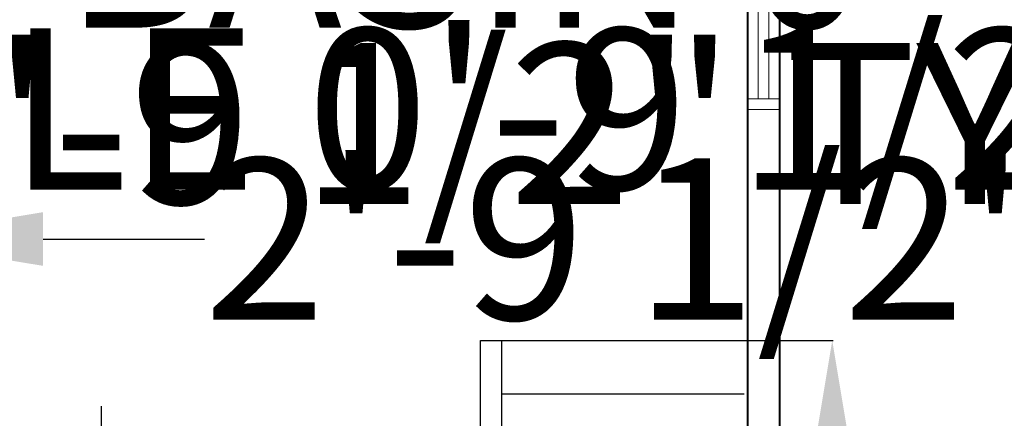
# Model space of a CAD drawing. Units: inches. Extents: x 7323 to 9737, y 2037 to 3322.
# Tile 13 of 19: x 9130 to 9314, y 2337 to 2411. Entities that reach past the tile are written whole.
import ezdxf

# ---------------------------------------------------------------- set-up
doc = ezdxf.new("R2010")
doc.units = ezdxf.units.IN
doc.header["$MEASUREMENT"] = 0
for name, color, linetype, lineweight in [('A-ANNO-DIMS', 2, 'Continuous', 18), ('A-FLOR-STRS', 7, 'Continuous', 25), ('A-GLAZ', 4, 'Continuous', 18), ('A-WALL', 7, 'Continuous', 40)]:
    doc.layers.add(name, color=color, linetype=linetype, lineweight=lineweight)
doc.styles.get("Standard").update_dxf_attribs({"font": 'arial.ttf'})
doc.dimstyles.get("Standard").update_dxf_attribs({"dimtxt": 30.18, "dimasz": 30.18, "dimexe": 0.18, "dimexo": 0.0625, "dimgap": 0.09, "dimtad": 0, "dimtih": 1, "dimtoh": 1, "dimdec": 0, "dimzin": 0, "dimdsep": 46, "dimlunit": 3, "dimtxsty": 'Standard', "dimcen": 0.09, "dimadec": 0, "dimazin": 0, "dimtfac": 1, "dimtdec": 0, "dimtofl": 0, "dimtmove": 0, "dimatfit": 3, "dimfxl": 1, "dimtolj": 1, "dimtzin": 0, "dimarcsym": 0})

# ---------------------------------------------------------------- blocks, each defined once
blk = doc.blocks.new('WIN-48')
for p, q in [((0, 0), (0, 6)), ((2, 0), (2, 6)), ((50, 0), (50, 6)), ((52, 0), (52, 6)), ((2, 4), (50, 4)), ((2, 2), (50, 2))]:
    blk.add_line(p, q)
blk = doc.blocks.new('STAIR-RETURN-FLIGHT')
for p, q in [((45.32, 110), (94.63, 110)), ((45.32, 0), (45.32, 110)), ((49.32, 0), (49.32, 110)), ((49.32, 100), (94.63, 100)), ((49.32, 90), (94.63, 90)), ((49.32, 80), (94.63, 80)), ((49.32, 70), (94.63, 70)), ((49.32, 60), (94.63, 60)), ((49.32, 50), (94.63, 50)), ((0, 40), (45.32, 40)), ((49.32, 40), (94.63, 40)), ((0, 30), (45.32, 30)), ((49.32, 30), (94.63, 30)), ((0, 20), (45.32, 20)), ((49.32, 20), (94.63, 20)), ((0, 10), (45.32, 10)), ((49.32, 10), (94.63, 10)), ((0, 0), (94.63, 0))]:
    blk.add_line(p, q)
blk = doc.blocks.new('*D41')
at = {"layer": 'A-ANNO-DIMS', "color": 0, "lineweight": -2, "transparency": 16777216}
for p, q in [((8661.59, 2428.04), (8661.59, 2458.22)), ((8661.59, 2458.22), (8691.77, 2458.22)), ((8657.46, 2397.86), (8661.77, 2397.86)), ((8657.46, 2369.86), (8661.77, 2369.86)), ((8661.59, 2339.68), (8661.59, 2309.5))]:
    blk.add_line(p, q, dxfattribs=at)
at = {"layer": 'A-ANNO-DIMS', "color": 0, "transparency": 16777216}
for points in [[(8656.56, 2428.04), (8666.62, 2428.04), (8661.59, 2397.86)], [(8656.56, 2339.68), (8666.62, 2339.68), (8661.59, 2369.86)]]:
    blk.add_solid(points, dxfattribs=at)
at = {"layer": 'Defpoints', "color": 0, "transparency": 16777216}
for p in [(8657.39, 2397.86), (8661.59, 2397.86), (8657.39, 2369.86)]:
    blk.add_point(p, dxfattribs=at)
at = {"layer": 'A-ANNO-DIMS', "color": 0, "transparency": 16777216, "insert": (8945.06, 2458.22), "char_height": 30.18, "attachment_point": 5}
blk.add_mtext('\\A1;VENT WINDOW 2\'-4" TYP.', dxfattribs=at)
blk = doc.blocks.new('*D43')
at = {"layer": 'A-ANNO-DIMS', "color": 0, "lineweight": -2, "transparency": 16777216}
for p, q in [((9108.94, 2438.75), (9108.94, 2468.93)), ((9104.01, 2408.57), (9109.12, 2408.57)), ((9104.01, 2375.3), (9109.12, 2375.3)), ((9108.94, 2345.12), (9108.94, 2314.94))]:
    blk.add_line(p, q, dxfattribs=at)
at = {"layer": 'A-ANNO-DIMS', "color": 0, "transparency": 16777216}
for points in [[(9103.91, 2438.75), (9113.97, 2438.75), (9108.94, 2408.57)], [(9103.91, 2345.12), (9113.97, 2345.12), (9108.94, 2375.3)]]:
    blk.add_solid(points, dxfattribs=at)
at = {"layer": 'Defpoints', "color": 0, "transparency": 16777216}
for p in [(9103.95, 2408.57), (9108.94, 2408.57), (9103.95, 2375.3)]:
    blk.add_point(p, dxfattribs=at)
at = {"layer": 'A-ANNO-DIMS', "color": 0, "transparency": 16777216, "insert": (9108.94, 2391.93), "char_height": 30.18, "attachment_point": 5}
blk.add_mtext('\\A1;BATH DOOR 2\'-9 1/2" TYP.', dxfattribs=at)
blk = doc.blocks.new('*D44')
at = {"layer": 'A-ANNO-DIMS', "color": 0, "lineweight": -2, "transparency": 16777216}
for p, q in [((9070.67, 2375.23), (9070.67, 2370.12)), ((9103.95, 2375.23), (9103.95, 2370.12)), ((9040.49, 2370.3), (9010.31, 2370.3)), ((9134.13, 2370.3), (9164.31, 2370.3))]:
    blk.add_line(p, q, dxfattribs=at)
at = {"layer": 'A-ANNO-DIMS', "color": 0, "transparency": 16777216}
for points in [[(9040.49, 2375.33), (9040.49, 2365.27), (9070.67, 2370.3)], [(9134.13, 2375.33), (9134.13, 2365.27), (9103.95, 2370.3)]]:
    blk.add_solid(points, dxfattribs=at)
at = {"layer": 'Defpoints', "color": 0, "transparency": 16777216}
for p in [(9070.67, 2375.3), (9103.95, 2375.3), (9103.95, 2370.3)]:
    blk.add_point(p, dxfattribs=at)
at = {"layer": 'A-ANNO-DIMS', "color": 0, "transparency": 16777216, "insert": (9291.8, 2370.3), "char_height": 30.18, "attachment_point": 5}
blk.add_mtext('\\A1;2\'-9 1/2" TYP.', dxfattribs=at)
blk = doc.blocks.new('*D47')
at = {"layer": 'A-ANNO-DIMS', "color": 0, "lineweight": -2, "transparency": 16777216}
for p, q in [((8809.55, 2464.49), (8779.37, 2464.49)), ((8839.73, 2461.79), (8839.73, 2464.67)), ((8858.14, 2461.79), (8858.14, 2464.67)), ((8888.32, 2464.49), (8918.5, 2464.49))]:
    blk.add_line(p, q, dxfattribs=at)
at = {"layer": 'A-ANNO-DIMS', "color": 0, "transparency": 16777216}
for points in [[(8809.55, 2469.52), (8809.55, 2459.46), (8839.73, 2464.49)], [(8888.32, 2469.52), (8888.32, 2459.46), (8858.14, 2464.49)]]:
    blk.add_solid(points, dxfattribs=at)
at = {"layer": 'Defpoints', "color": 0, "transparency": 16777216}
for p in [(8858.14, 2464.49), (8839.73, 2461.73), (8858.14, 2461.73)]:
    blk.add_point(p, dxfattribs=at)
at = {"layer": 'A-ANNO-DIMS', "color": 0, "transparency": 16777216, "insert": (9164.9, 2464.49), "char_height": 30.18, "attachment_point": 5}
blk.add_mtext('\\A1;ARMCHAIR 1\'-6 1/2" TYP.', dxfattribs=at)
blk = doc.blocks.new('*D51')
at = {"layer": 'A-ANNO-DIMS', "color": 0, "lineweight": -2, "transparency": 16777216}
for p, q in [((9130.95, 2513.23), (9130.95, 2501.42)), ((9208.95, 2513.23), (9208.95, 2501.42)), ((9161.13, 2501.6), (9178.77, 2501.6)), ((9208.95, 2501.6), (9239.13, 2501.6))]:
    blk.add_line(p, q, dxfattribs=at)
at = {"layer": 'A-ANNO-DIMS', "color": 0, "transparency": 16777216}
for points in [[(9161.13, 2506.63), (9161.13, 2496.57), (9130.95, 2501.6)], [(9178.77, 2506.63), (9178.77, 2496.57), (9208.95, 2501.6)]]:
    blk.add_solid(points, dxfattribs=at)
at = {"layer": 'Defpoints', "color": 0, "transparency": 16777216}
for p in [(9130.95, 2513.3), (9208.95, 2513.3), (9208.95, 2501.6)]:
    blk.add_point(p, dxfattribs=at)
at = {"layer": 'A-ANNO-DIMS', "color": 0, "transparency": 16777216, "insert": (9492.09, 2501.6), "char_height": 30.18, "attachment_point": 5}
blk.add_mtext('\\A1;DOUBLE DOOR 6\'-6" TYP.', dxfattribs=at)
blk = doc.blocks.new('*D55')
at = {"layer": 'A-ANNO-DIMS', "color": 0, "lineweight": -2, "transparency": 16777216}
for p, q in [((9265.38, 2351.3), (9282, 2351.3)), ((9281.82, 2321.12), (9281.82, 2311.99)), ((9281.82, 2271.48), (9281.82, 2280.6)), ((9265.38, 2241.3), (9282, 2241.3))]:
    blk.add_line(p, q, dxfattribs=at)
at = {"layer": 'A-ANNO-DIMS', "color": 0, "transparency": 16777216}
for points in [[(9276.79, 2321.12), (9286.85, 2321.12), (9281.82, 2351.3)], [(9276.79, 2271.48), (9286.85, 2271.48), (9281.82, 2241.3)]]:
    blk.add_solid(points, dxfattribs=at)
at = {"layer": 'Defpoints', "color": 0, "transparency": 16777216}
for p in [(9265.32, 2351.3), (9281.82, 2351.3), (9265.32, 2241.3)]:
    blk.add_point(p, dxfattribs=at)
at = {"layer": 'A-ANNO-DIMS', "color": 0, "transparency": 16777216, "insert": (9281.82, 2296.3), "char_height": 30.18, "attachment_point": 5}
blk.add_mtext('\\A1;STAIR FLIGHT 9\'-2" TYP.', dxfattribs=at)
blk = doc.blocks.new('*D59')
at = {"layer": 'A-ANNO-DIMS', "color": 0, "lineweight": -2, "transparency": 16777216}
for p, q in [((9064.67, 2473.96), (9064.67, 2467.95)), ((9103.95, 2473.96), (9103.95, 2467.95)), ((9034.49, 2468.13), (9004.31, 2468.13)), ((9134.13, 2468.13), (9164.31, 2468.13))]:
    blk.add_line(p, q, dxfattribs=at)
at = {"layer": 'A-ANNO-DIMS', "color": 0, "transparency": 16777216}
for points in [[(9034.49, 2473.16), (9034.49, 2463.1), (9064.67, 2468.13)], [(9134.13, 2473.16), (9134.13, 2463.1), (9103.95, 2468.13)]]:
    blk.add_solid(points, dxfattribs=at)
at = {"layer": 'Defpoints', "color": 0, "transparency": 16777216}
for p in [(9064.67, 2474.02), (9103.95, 2474.02), (9103.95, 2468.13)]:
    blk.add_point(p, dxfattribs=at)
at = {"layer": 'A-ANNO-DIMS', "color": 0, "transparency": 16777216, "insert": (9458.35, 2468.13), "char_height": 30.18, "attachment_point": 5}
blk.add_mtext('\\A1;KITCHEN DOOR 3\'-3 1/2" TYP.', dxfattribs=at)
blk = doc.blocks.new('*D63')
at = {"layer": 'A-ANNO-DIMS', "color": 0, "lineweight": -2, "transparency": 16777216}
for p, q in [((8744.72, 2466.22), (8744.72, 2496.4)), ((8744.72, 2496.4), (8774.9, 2496.4)), ((8741.46, 2436.04), (8744.9, 2436.04)), ((8741.46, 2413.86), (8744.9, 2413.86)), ((8744.72, 2383.68), (8744.72, 2353.5))]:
    blk.add_line(p, q, dxfattribs=at)
at = {"layer": 'A-ANNO-DIMS', "color": 0, "transparency": 16777216}
for points in [[(8739.69, 2466.22), (8749.75, 2466.22), (8744.72, 2436.04)], [(8739.69, 2383.68), (8749.75, 2383.68), (8744.72, 2413.86)]]:
    blk.add_solid(points, dxfattribs=at)
at = {"layer": 'Defpoints', "color": 0, "transparency": 16777216}
for p in [(8741.39, 2436.04), (8744.72, 2436.04), (8741.39, 2413.86)]:
    blk.add_point(p, dxfattribs=at)
at = {"layer": 'A-ANNO-DIMS', "color": 0, "transparency": 16777216, "insert": (9003.76, 2496.4), "char_height": 30.18, "attachment_point": 5}
blk.add_mtext('\\A1;APPLIANCE 1\'-10" TYP.', dxfattribs=at)
blk = doc.blocks.new('*D67')
at = {"layer": 'A-ANNO-DIMS', "color": 0, "lineweight": -2, "transparency": 16777216}
for p, q in [((9145.07, 2308.82), (9145.07, 2339)), ((9150.37, 2278.64), (9144.89, 2278.64)), ((9150.37, 2242.89), (9144.89, 2242.89)), ((9145.07, 2212.71), (9145.07, 2182.53))]:
    blk.add_line(p, q, dxfattribs=at)
at = {"layer": 'A-ANNO-DIMS', "color": 0, "transparency": 16777216}
for points in [[(9140.04, 2308.82), (9150.1, 2308.82), (9145.07, 2278.64)], [(9140.04, 2212.71), (9150.1, 2212.71), (9145.07, 2242.89)]]:
    blk.add_solid(points, dxfattribs=at)
at = {"layer": 'Defpoints', "color": 0, "transparency": 16777216}
for p in [(9145.07, 2278.64), (9150.44, 2278.64), (9150.44, 2242.89)]:
    blk.add_point(p, dxfattribs=at)
at = {"layer": 'A-ANNO-DIMS', "color": 0, "transparency": 16777216, "insert": (9145.07, 2260.76), "char_height": 30.18, "attachment_point": 5}
blk.add_mtext('\\A1;TV UNIT 2\'-11 1/2" TYP.', dxfattribs=at)
blk = doc.blocks.new('*D68')
at = {"layer": 'A-ANNO-DIMS', "color": 0, "lineweight": -2, "transparency": 16777216}
for p, q in [((9120.26, 2284), (9090.08, 2284)), ((9150.44, 2278.7), (9150.44, 2284.18)), ((9163.95, 2278.7), (9163.95, 2284.18)), ((9194.13, 2284), (9224.31, 2284))]:
    blk.add_line(p, q, dxfattribs=at)
at = {"layer": 'A-ANNO-DIMS', "color": 0, "transparency": 16777216}
for points in [[(9120.26, 2289.03), (9120.26, 2278.97), (9150.44, 2284)], [(9194.13, 2289.03), (9194.13, 2278.97), (9163.95, 2284)]]:
    blk.add_solid(points, dxfattribs=at)
at = {"layer": 'Defpoints', "color": 0, "transparency": 16777216}
for p in [(9163.95, 2284), (9150.44, 2278.64), (9163.95, 2278.64)]:
    blk.add_point(p, dxfattribs=at)
at = {"layer": 'A-ANNO-DIMS', "color": 0, "transparency": 16777216, "insert": (9350.12, 2284), "char_height": 30.18, "attachment_point": 5}
blk.add_mtext('\\A1;1\'-1 1/2" TYP.', dxfattribs=at)
blk = doc.blocks.new('*D69')
at = {"layer": 'A-ANNO-DIMS', "color": 0, "lineweight": -2, "transparency": 16777216}
for p, q in [((8836.58, 2472.89), (8836.58, 2503.07)), ((8836.58, 2503.07), (8866.76, 2503.07)), ((8839.88, 2442.71), (8836.4, 2442.71)), ((8839.88, 2420.33), (8836.4, 2420.33)), ((8836.58, 2390.15), (8836.58, 2359.97))]:
    blk.add_line(p, q, dxfattribs=at)
at = {"layer": 'A-ANNO-DIMS', "color": 0, "transparency": 16777216}
for points in [[(8831.55, 2472.89), (8841.61, 2472.89), (8836.58, 2442.71)], [(8831.55, 2390.15), (8841.61, 2390.15), (8836.58, 2420.33)]]:
    blk.add_solid(points, dxfattribs=at)
at = {"layer": 'Defpoints', "color": 0, "transparency": 16777216}
for p in [(8836.58, 2442.71), (8839.94, 2442.71), (8839.94, 2420.33)]:
    blk.add_point(p, dxfattribs=at)
at = {"layer": 'A-ANNO-DIMS', "color": 0, "transparency": 16777216, "insert": (9169.54, 2503.07), "char_height": 30.18, "attachment_point": 5}
blk.add_mtext('\\A1;COFFEE TABLE 1\'-10 1/2" TYP.', dxfattribs=at)
blk = doc.blocks.new('*D73')
at = {"layer": 'A-ANNO-DIMS', "color": 0, "lineweight": -2, "transparency": 16777216}
for p, q in [((9061.59, 2423.36), (9061.59, 2425.15)), ((9072.75, 2423.36), (9072.75, 2425.15)), ((9031.41, 2424.97), (9001.23, 2424.97)), ((9102.93, 2424.97), (9133.11, 2424.97))]:
    blk.add_line(p, q, dxfattribs=at)
at = {"layer": 'A-ANNO-DIMS', "color": 0, "transparency": 16777216}
for points in [[(9031.41, 2430), (9031.41, 2419.94), (9061.59, 2424.97)], [(9102.93, 2430), (9102.93, 2419.94), (9072.75, 2424.97)]]:
    blk.add_solid(points, dxfattribs=at)
at = {"layer": 'Defpoints', "color": 0, "transparency": 16777216}
for p in [(9061.59, 2423.3), (9072.75, 2424.97), (9072.75, 2423.3)]:
    blk.add_point(p, dxfattribs=at)
at = {"layer": 'A-ANNO-DIMS', "color": 0, "transparency": 16777216, "insert": (9305.36, 2424.97), "char_height": 30.18, "attachment_point": 5}
blk.add_mtext('\\A1;BASIN 0\'-11" TYP.', dxfattribs=at)
blk = doc.blocks.new('*D74')
at = {"layer": 'A-ANNO-DIMS', "color": 0, "lineweight": -2, "transparency": 16777216}
for p, q in [((9059.91, 2453.48), (9059.91, 2483.66)), ((9059.91, 2483.66), (9090.09, 2483.66)), ((9061.53, 2423.3), (9059.73, 2423.3)), ((9061.53, 2413.24), (9059.73, 2413.24)), ((9059.91, 2383.06), (9059.91, 2352.88))]:
    blk.add_line(p, q, dxfattribs=at)
at = {"layer": 'A-ANNO-DIMS', "color": 0, "transparency": 16777216}
for points in [[(9054.88, 2453.48), (9064.94, 2453.48), (9059.91, 2423.3)], [(9054.88, 2383.06), (9064.94, 2383.06), (9059.91, 2413.24)]]:
    blk.add_solid(points, dxfattribs=at)
at = {"layer": 'Defpoints', "color": 0, "transparency": 16777216}
for p in [(9059.91, 2423.3), (9061.59, 2423.3), (9061.59, 2413.24)]:
    blk.add_point(p, dxfattribs=at)
at = {"layer": 'A-ANNO-DIMS', "color": 0, "transparency": 16777216, "insert": (9193.89, 2483.66), "char_height": 30.18, "attachment_point": 5}
blk.add_mtext('\\A1;0\'-10" TYP.', dxfattribs=at)
blk = doc.blocks.new('*D75')
at = {"layer": 'A-ANNO-DIMS', "color": 0, "lineweight": -2, "transparency": 16777216}
for p, q in [((8629.63, 2293.84), (8599.45, 2293.84)), ((8659.81, 2292), (8659.81, 2294.02)), ((8672.52, 2292), (8672.52, 2294.02)), ((8702.7, 2293.84), (8732.88, 2293.84))]:
    blk.add_line(p, q, dxfattribs=at)
at = {"layer": 'A-ANNO-DIMS', "color": 0, "transparency": 16777216}
for points in [[(8629.63, 2298.87), (8629.63, 2288.81), (8659.81, 2293.84)], [(8702.7, 2298.87), (8702.7, 2288.81), (8672.52, 2293.84)]]:
    blk.add_solid(points, dxfattribs=at)
at = {"layer": 'Defpoints', "color": 0, "transparency": 16777216}
for p in [(8672.52, 2293.84), (8659.81, 2291.93), (8672.52, 2291.93)]:
    blk.add_point(p, dxfattribs=at)
at = {"layer": 'A-ANNO-DIMS', "color": 0, "transparency": 16777216, "insert": (9002.27, 2293.84), "char_height": 30.18, "attachment_point": 5}
blk.add_mtext('\\A1;NIGHTSTAND 1\'-0 1/2" TYP.', dxfattribs=at)
blk = doc.blocks.new('*D78')
at = {"layer": 'A-ANNO-DIMS', "color": 0, "lineweight": -2, "transparency": 16777216}
for p, q in [((9030.98, 2259.48), (9030.98, 2289.66)), ((9030.98, 2289.66), (9061.16, 2289.66)), ((9029.14, 2229.3), (9031.16, 2229.3)), ((9029.14, 2219.69), (9031.16, 2219.69)), ((9030.98, 2189.51), (9030.98, 2159.33))]:
    blk.add_line(p, q, dxfattribs=at)
at = {"layer": 'A-ANNO-DIMS', "color": 0, "transparency": 16777216}
for points in [[(9025.95, 2259.48), (9036.01, 2259.48), (9030.98, 2229.3)], [(9025.95, 2189.51), (9036.01, 2189.51), (9030.98, 2219.69)]]:
    blk.add_solid(points, dxfattribs=at)
at = {"layer": 'Defpoints', "color": 0, "transparency": 16777216}
for p in [(9029.07, 2229.3), (9030.98, 2229.3), (9029.07, 2219.69)]:
    blk.add_point(p, dxfattribs=at)
at = {"layer": 'A-ANNO-DIMS', "color": 0, "transparency": 16777216, "insert": (9188.39, 2289.66), "char_height": 30.18, "attachment_point": 5}
blk.add_mtext('\\A1;0\'-9 1/2" TYP.', dxfattribs=at)
blk = doc.blocks.new('*D79')
at = {"layer": 'A-ANNO-DIMS', "color": 0, "lineweight": -2, "transparency": 16777216}
for p, q in [((8871.1, 2395.97), (8871.1, 2394.46)), ((8880.36, 2395.97), (8880.36, 2394.46)), ((8840.92, 2394.64), (8810.74, 2394.64)), ((8910.54, 2394.64), (8940.72, 2394.64))]:
    blk.add_line(p, q, dxfattribs=at)
at = {"layer": 'A-ANNO-DIMS', "color": 0, "transparency": 16777216}
for points in [[(8840.92, 2399.67), (8840.92, 2389.61), (8871.1, 2394.64)], [(8910.54, 2399.67), (8910.54, 2389.61), (8880.36, 2394.64)]]:
    blk.add_solid(points, dxfattribs=at)
at = {"layer": 'Defpoints', "color": 0, "transparency": 16777216}
for p in [(8871.1, 2396.03), (8880.36, 2396.03), (8880.36, 2394.64)]:
    blk.add_point(p, dxfattribs=at)
at = {"layer": 'A-ANNO-DIMS', "color": 0, "transparency": 16777216, "insert": (9195.57, 2394.64), "char_height": 30.18, "attachment_point": 5}
blk.add_mtext('\\A1;SIDE TABLE 0\'-9 1/2" TYP.', dxfattribs=at)
blk = doc.blocks.new('*D105')
at = {"layer": 'A-ANNO-DIMS', "color": 0, "lineweight": -2, "transparency": 16777216}
for p, q in [((9007.945402, 2365.232705), (9007.945402, 2148.482809)), ((9103.945402, 2333.232705), (9103.945402, 2148.482809)), ((8977.765402, 2148.662809), (8947.585402, 2148.662809)), ((9134.125402, 2148.662809), (9164.305402, 2148.662809))]:
    blk.add_line(p, q, dxfattribs=at)
at = {"layer": 'A-ANNO-DIMS', "color": 0, "transparency": 16777216}
for points in [[(8977.765402, 2153.692809), (8977.765402, 2143.632809), (9007.945402, 2148.662809)], [(9134.125402, 2153.692809), (9134.125402, 2143.632809), (9103.945402, 2148.662809)]]:
    blk.add_solid(points, dxfattribs=at)
at = {"layer": 'Defpoints', "color": 0, "transparency": 16777216}
for p in [(9007.945402, 2365.295205), (9103.945402, 2333.295205), (9103.945402, 2148.662809)]:
    blk.add_point(p, dxfattribs=at)
at = {"layer": 'A-ANNO-DIMS', "color": 0, "transparency": 16777216, "insert": (9055.945402, 2148.662809), "char_height": 30.18, "attachment_point": 5}
blk.add_mtext('\\A1;8\'-0"', dxfattribs=at)
blk = doc.blocks.new('*D109')
at = {"layer": 'A-ANNO-DIMS', "color": 0, "lineweight": -2, "transparency": 16777216}
for p, q in [((9016.91, 2377.23), (9016.91, 2148.48)), ((9034.93, 2377.23), (9034.93, 2148.48)), ((8986.73, 2148.66), (8956.55, 2148.66)), ((9065.11, 2148.66), (9095.29, 2148.66))]:
    blk.add_line(p, q, dxfattribs=at)
at = {"layer": 'A-ANNO-DIMS', "color": 0, "transparency": 16777216}
for points in [[(8986.73, 2153.69), (8986.73, 2143.63), (9016.91, 2148.66)], [(9065.11, 2153.69), (9065.11, 2143.63), (9034.93, 2148.66)]]:
    blk.add_solid(points, dxfattribs=at)
at = {"layer": 'Defpoints', "color": 0, "transparency": 16777216}
for p in [(9016.91, 2377.3), (9034.93, 2377.3), (9034.93, 2148.66)]:
    blk.add_point(p, dxfattribs=at)
at = {"layer": 'A-ANNO-DIMS', "color": 0, "transparency": 16777216, "insert": (9134.07, 2148.66), "char_height": 30.18, "attachment_point": 5}
blk.add_mtext('\\A1;1\'-6"', dxfattribs=at)

msp = doc.modelspace()

# ---------------------------------------------------------------- linework, layer by layer
at = {"layer": 'A-WALL'}
for p, q in [((9271.95, 2687.3), (9271.95, 2199.3)), ((9265.95, 2513.3), (9265.95, 2205.3))]:
    msp.add_line(p, q, dxfattribs=at)

# ---------------------------------------------------------------- block references
at = {"layer": 'A-FLOR-STRS'}
msp.add_blockref('STAIR-RETURN-FLIGHT', (9170.68, 2241.3), dxfattribs=at)
at = {"layer": 'A-GLAZ', "rotation": 270.000000000004}
msp.add_blockref('WIN-48', (9265.95, 2446.56), dxfattribs=at)

# ---------------------------------------------------------------- dimensions: what is measured, and where the dimension line sits
at = {"layer": 'A-ANNO-DIMS'}
for base, p1, p2, text, picture, middle in [((8836.58, 2442.71), (8839.94, 2420.33), (8839.94, 2442.71), 'COFFEE TABLE <> TYP.', '*D69', (9169.54, 2503.07)), ((8744.72, 2436.04), (8741.39, 2413.86), (8741.39, 2436.04), 'APPLIANCE <> TYP.', '*D63', (9003.76, 2496.4)), ((8661.59, 2397.86), (8657.39, 2369.86), (8657.39, 2397.86), 'VENT WINDOW <> TYP.', '*D41', (8945.06, 2458.22)), ((9059.91, 2423.3), (9061.59, 2413.24), (9061.59, 2423.3), '<> TYP.', '*D74', (9193.89, 2483.66)), ((9108.94, 2408.57), (9103.95, 2375.3), (9103.95, 2408.57), 'BATH DOOR <> TYP.', '*D43', (9108.94, 2391.93)), ((9281.82, 2351.3), (9265.32, 2241.3), (9265.32, 2351.3), 'STAIR FLIGHT <> TYP.', '*D55', (9281.82, 2296.3)), ((9145.0746, 2278.635), (9150.4365, 2242.8889), (9150.4365, 2278.635), 'TV UNIT <> TYP.', '*D67', (9145.0746, 2260.762)), ((9030.98, 2229.3), (9029.07, 2219.69), (9029.07, 2229.3), '<> TYP.', '*D78', (9188.39, 2289.66))]:
    dim = msp.add_linear_dim(base=base, p1=p1, p2=p2, angle=90, text=text, dimstyle='Standard', override={"dimdec": 1, "dimlfac": 1, "dimrnd": 0, "dimzin": 1, "dimdsep": 46, "dimlunit": 4, "dimfrac": 2}, dxfattribs=at)
    dim.commit()
    dim.dimension.update_dxf_attribs({"geometry": picture, "text_midpoint": middle})
for base, p1, p2, text, picture, middle in [((9208.95, 2501.6), (9130.95, 2513.3), (9208.95, 2513.3), 'DOUBLE DOOR <> TYP.', '*D51', (9492.09, 2501.6)), ((9103.95, 2468.13), (9064.67, 2474.02), (9103.95, 2474.02), 'KITCHEN DOOR <> TYP.', '*D59', (9458.35, 2468.13)), ((8858.14, 2464.49), (8839.73, 2461.73), (8858.14, 2461.73), 'ARMCHAIR <> TYP.', '*D47', (9164.9, 2464.49)), ((8880.36, 2394.64), (8871.1, 2396.03), (8880.36, 2396.03), 'SIDE TABLE <> TYP.', '*D79', (9195.57, 2394.64)), ((9072.75, 2424.97), (9061.59, 2423.3), (9072.75, 2423.3), 'BASIN <> TYP.', '*D73', (9305.36, 2424.97)), ((9103.95, 2370.3), (9070.67, 2375.3), (9103.95, 2375.3), '<> TYP.', '*D44', (9291.8, 2370.3)), ((8672.52, 2293.84), (8659.81, 2291.93), (8672.52, 2291.93), 'NIGHTSTAND <> TYP.', '*D75', (9002.27, 2293.84)), ((9163.95, 2284), (9150.44, 2278.64), (9163.95, 2278.64), '<> TYP.', '*D68', (9350.12, 2284))]:
    dim = msp.add_linear_dim(base=base, p1=p1, p2=p2, text=text, dimstyle='Standard', override={"dimdec": 1, "dimlfac": 1, "dimrnd": 0, "dimzin": 1, "dimdsep": 46, "dimlunit": 4, "dimfrac": 2}, dxfattribs=at)
    dim.commit()
    dim.dimension.update_dxf_attribs({"geometry": picture, "text_midpoint": middle})
for base, p1, p2, picture, middle in [((9034.93, 2148.66), (9016.91, 2377.3), (9034.93, 2377.3), '*D109', (9134.07, 2148.66)), ((9103.95, 2148.66), (9007.95, 2365.3), (9103.95, 2333.3), '*D105', (9055.95, 2148.66))]:
    dim = msp.add_linear_dim(base=base, p1=p1, p2=p2, dimstyle='Standard', override={"dimdec": 1, "dimlfac": 1, "dimrnd": 0, "dimzin": 1, "dimdsep": 46, "dimlunit": 4, "dimfrac": 2}, dxfattribs=at)
    dim.commit()
    dim.dimension.update_dxf_attribs({"geometry": picture, "text_midpoint": middle})

doc.saveas('drawing.dxf')
